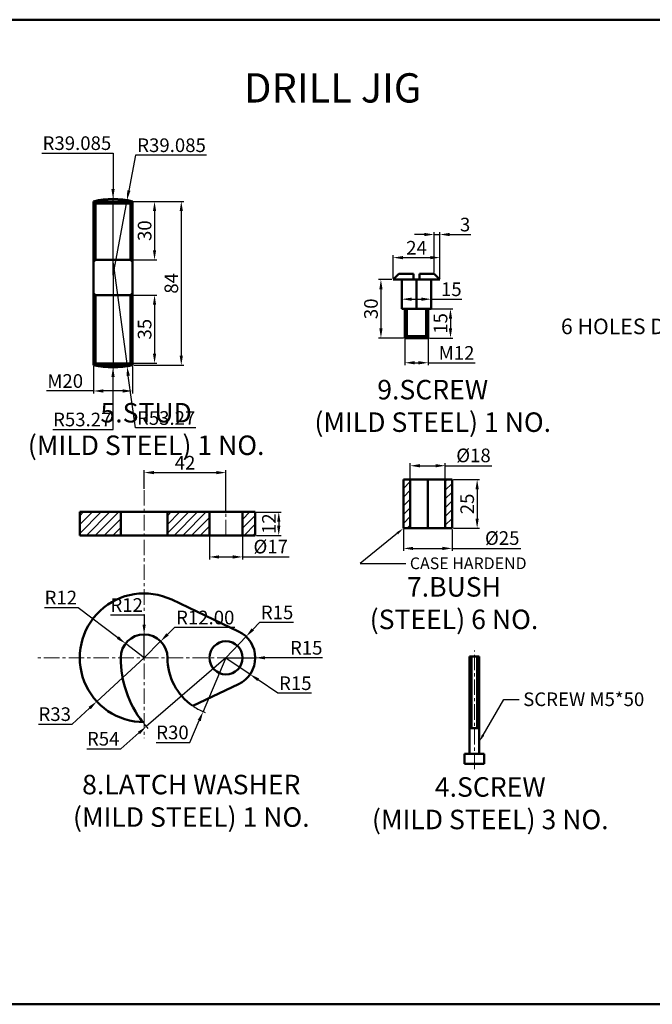
# Model space of a CAD drawing. Units: millimetres. Extents: x 51 to 972, y -225 to 280.
# Tile 2 of 3: x 270 to 594, y -225 to 280. Entities that reach past the tile are written whole.
import ezdxf
from ezdxf import colors
from ezdxf.entities.mleader import LeaderData, LeaderLine
from ezdxf.math import Vec2, Vec3

# ---------------------------------------------------------------- set-up
doc = ezdxf.new("R2010")
doc.units = ezdxf.units.MM
doc.header["$LTSCALE"] = 0.5
doc.linetypes.add('CENTER', pattern=[50.8, 31.75, -6.35, 6.35, -6.35])
for name, color, linetype, lineweight in [('M-CNTR', 1, 'CENTER', 18), ('M-DIMS', 2, 'Continuous', 25), ('M-HATC', 8, 'Continuous', 18), ('M-OUTL', 7, 'Continuous', 50), ('M-TEXT', 7, 'Continuous', 25), ('M-TTLB', 7, 'Continuous', 50)]:
    doc.layers.add(name, color=color, linetype=linetype, lineweight=lineweight)
doc.styles.get("Standard").update_dxf_attribs({"font": 'arial.ttf'})
doc.dimstyles.new('ISO-25', dxfattribs={"dimtxt": 7, "dimasz": 5, "dimexe": 1.25, "dimexo": 0.625, "dimtad": 1, "dimtoh": 1, "dimtxsty": 'Standard', "dimcen": 2.5, "dimadec": 0, "dimazin": 0, "dimtfac": 1, "dimtmove": 0, "dimatfit": 3, "dimfxl": 1, "dimarcsym": 0})

# ---------------------------------------------------------------- blocks, each defined once
blk = doc.blocks.new('*D9')
at = {"layer": 'Defpoints', "color": 0, "ltscale": 0.5, "transparency": 16777216}
for p in [(327.79, 186.58), (327.79, 102.58), (352.8, 102.58)]:
    blk.add_point(p, dxfattribs=at)
at = {"layer": 'M-DIMS', "color": 0, "lineweight": -2, "ltscale": 0.5, "transparency": 16777216}
for p, q in [((328.41, 186.58), (354.05, 186.58)), ((352.8, 181.58), (352.8, 107.58)), ((328.41, 102.58), (354.05, 102.58))]:
    blk.add_line(p, q, dxfattribs=at)
at = {"layer": 'M-DIMS', "color": 0, "ltscale": 0.5, "transparency": 16777216}
for points in [[(351.96, 181.58), (353.63, 181.58), (352.8, 186.58)], [(351.96, 107.58), (353.63, 107.58), (352.8, 102.58)]]:
    blk.add_solid(points, dxfattribs=at)
at = {"layer": 'M-DIMS', "color": 0, "ltscale": 0.5, "transparency": 16777216, "insert": (348.6, 144.58), "char_height": 7, "attachment_point": 5, "rotation": 90}
blk.add_mtext('84', dxfattribs=at)
blk = doc.blocks.new('*D10')
at = {"layer": 'Defpoints', "color": 0, "ltscale": 0.5, "transparency": 16777216}
for p in [(324.33, 138.58), (321.83, 103.58), (339.08, 103.58)]:
    blk.add_point(p, dxfattribs=at)
at = {"layer": 'M-DIMS', "color": 0, "lineweight": -2, "ltscale": 0.5, "transparency": 16777216}
for p, q in [((324.96, 138.58), (340.33, 138.58)), ((339.08, 133.58), (339.08, 108.58)), ((322.46, 103.58), (340.33, 103.58))]:
    blk.add_line(p, q, dxfattribs=at)
at = {"layer": 'M-DIMS', "color": 0, "ltscale": 0.5, "transparency": 16777216}
for points in [[(338.25, 133.58), (339.91, 133.58), (339.08, 138.58)], [(338.25, 108.58), (339.91, 108.58), (339.08, 103.58)]]:
    blk.add_solid(points, dxfattribs=at)
at = {"layer": 'M-DIMS', "color": 0, "ltscale": 0.5, "transparency": 16777216, "insert": (334.88, 121.08), "char_height": 7, "attachment_point": 5, "rotation": 90}
blk.add_mtext('35', dxfattribs=at)
blk = doc.blocks.new('*D11')
at = {"layer": 'Defpoints', "color": 0, "ltscale": 0.5, "transparency": 16777216}
for p in [(317.79, 186.58), (317.79, 156.58), (339.08, 156.58)]:
    blk.add_point(p, dxfattribs=at)
at = {"layer": 'M-DIMS', "color": 0, "lineweight": -2, "ltscale": 0.5, "transparency": 16777216}
for p, q in [((318.41, 186.58), (340.33, 186.58)), ((339.08, 181.58), (339.08, 161.58)), ((318.41, 156.58), (340.33, 156.58))]:
    blk.add_line(p, q, dxfattribs=at)
at = {"layer": 'M-DIMS', "color": 0, "ltscale": 0.5, "transparency": 16777216}
for points in [[(338.25, 181.58), (339.91, 181.58), (339.08, 186.58)], [(338.25, 161.58), (339.91, 161.58), (339.08, 156.58)]]:
    blk.add_solid(points, dxfattribs=at)
at = {"layer": 'M-DIMS', "color": 0, "ltscale": 0.5, "transparency": 16777216, "insert": (334.88, 171.58), "char_height": 7, "attachment_point": 5, "rotation": 90}
blk.add_mtext('30', dxfattribs=at)
blk = doc.blocks.new('*D12')
at = {"layer": 'Defpoints', "color": 0, "ltscale": 0.5, "transparency": 16777216}
for p in [(307.79, 102.58), (327.79, 102.58), (327.79, 89.41)]:
    blk.add_point(p, dxfattribs=at)
at = {"layer": 'M-DIMS', "color": 0, "lineweight": -2, "ltscale": 0.5, "transparency": 16777216}
for p, q in [((307.79, 101.95), (307.79, 88.16)), ((327.79, 101.95), (327.79, 88.16)), ((307.79, 89.41), (283.71, 89.41)), ((322.79, 89.41), (312.79, 89.41))]:
    blk.add_line(p, q, dxfattribs=at)
at = {"layer": 'M-DIMS', "color": 0, "ltscale": 0.5, "transparency": 16777216}
for points in [[(312.79, 90.24), (312.79, 88.57), (307.79, 89.41)], [(322.79, 90.24), (322.79, 88.57), (327.79, 89.41)]]:
    blk.add_solid(points, dxfattribs=at)
at = {"layer": 'M-DIMS', "color": 0, "ltscale": 0.5, "transparency": 16777216, "insert": (293.25, 93.61), "char_height": 7, "attachment_point": 5}
blk.add_mtext('M20', dxfattribs=at)
blk = doc.blocks.new('*D13')
at = {"layer": 'Defpoints', "color": 0, "ltscale": 0.5, "transparency": 16777216}
for p in [(375.73, -47.35), (388.11, -55.82)]:
    blk.add_point(p, dxfattribs=at)
at = {"layer": 'M-DIMS', "color": 0, "lineweight": -2, "ltscale": 0.5, "transparency": 16777216}
for p, q in [((375.73, -47.35), (388.11, -55.82)), ((402.26, -65.5), (392.23, -58.64)), ((419.67, -65.5), (402.26, -65.5))]:
    blk.add_line(p, q, dxfattribs=at)
at = {"layer": 'M-DIMS', "color": 0, "ltscale": 0.5, "transparency": 16777216}
blk.add_solid([(392.71, -57.96), (391.76, -59.33), (388.11, -55.82)], dxfattribs=at)
at = {"layer": 'M-DIMS', "color": 0, "ltscale": 0.5, "transparency": 16777216, "insert": (411.28, -61.3), "char_height": 7, "attachment_point": 5}
blk.add_mtext('R15', dxfattribs=at)
blk = doc.blocks.new('*D14')
at = {"layer": 'Defpoints', "color": 0, "ltscale": 0.5, "transparency": 16777216}
for p in [(324.19, -40.06), (333.73, -47.35)]:
    blk.add_point(p, dxfattribs=at)
at = {"layer": 'M-DIMS', "color": 0, "lineweight": -2, "ltscale": 0.5, "transparency": 16777216}
for p, q in [((282.68, -21.53), (299.96, -21.53)), ((299.96, -21.53), (320.22, -37.03)), ((333.73, -47.35), (324.19, -40.06))]:
    blk.add_line(p, q, dxfattribs=at)
at = {"layer": 'M-DIMS', "color": 0, "ltscale": 0.5, "transparency": 16777216}
blk.add_solid([(320.73, -36.36), (319.72, -37.69), (324.19, -40.06)], dxfattribs=at)
at = {"layer": 'M-DIMS', "color": 0, "ltscale": 0.5, "transparency": 16777216, "insert": (291.01, -17.39), "char_height": 7, "attachment_point": 5}
blk.add_mtext('R12', dxfattribs=at)
blk = doc.blocks.new('*D15')
at = {"layer": 'Defpoints', "color": 0, "ltscale": 0.5, "transparency": 16777216}
for p in [(333.73, -47.35), (309.47, -69.73)]:
    blk.add_point(p, dxfattribs=at)
at = {"layer": 'M-DIMS', "color": 0, "lineweight": -2, "ltscale": 0.5, "transparency": 16777216}
for p, q in [((333.73, -47.35), (309.47, -69.73)), ((296.86, -81.36), (305.8, -73.12)), ((279.51, -81.36), (296.86, -81.36))]:
    blk.add_line(p, q, dxfattribs=at)
at = {"layer": 'M-DIMS', "color": 0, "ltscale": 0.5, "transparency": 16777216}
blk.add_solid([(305.23, -72.51), (306.36, -73.73), (309.47, -69.73)], dxfattribs=at)
at = {"layer": 'M-DIMS', "color": 0, "ltscale": 0.5, "transparency": 16777216, "insert": (287.88, -77.16), "char_height": 7, "attachment_point": 5}
blk.add_mtext('R33', dxfattribs=at)
blk = doc.blocks.new('*D16')
at = {"layer": 'Defpoints', "color": 0, "ltscale": 0.5, "transparency": 16777216}
for p in [(375.73, -47.35), (363.97, -74.95)]:
    blk.add_point(p, dxfattribs=at)
at = {"layer": 'M-DIMS', "color": 0, "lineweight": -2, "ltscale": 0.5, "transparency": 16777216}
for p, q in [((375.73, -47.35), (363.97, -74.95)), ((357.25, -90.73), (362.01, -79.55)), ((339.92, -90.73), (357.25, -90.73))]:
    blk.add_line(p, q, dxfattribs=at)
blk.add_arc((375.73, -47.35), 30, 236.5706, 249.317, dxfattribs=at)
at = {"layer": 'M-DIMS', "color": 0, "ltscale": 0.5, "transparency": 16777216}
blk.add_solid([(361.24, -79.23), (362.78, -79.88), (363.97, -74.95)], dxfattribs=at)
at = {"layer": 'M-DIMS', "color": 0, "ltscale": 0.5, "transparency": 16777216, "insert": (348.27, -86.53), "char_height": 7, "attachment_point": 5}
blk.add_mtext('R30', dxfattribs=at)
blk = doc.blocks.new('*D17')
at = {"layer": 'Defpoints', "color": 0, "ltscale": 0.5, "transparency": 16777216}
for p in [(375.73, -47.35), (334.84, -82.63)]:
    blk.add_point(p, dxfattribs=at)
at = {"layer": 'M-DIMS', "color": 0, "lineweight": -2, "ltscale": 0.5, "transparency": 16777216}
for p, q in [((375.73, -47.35), (334.84, -82.63)), ((321.72, -93.95), (331.06, -85.9)), ((304.4, -93.95), (321.72, -93.95))]:
    blk.add_line(p, q, dxfattribs=at)
blk.add_arc((375.73, -47.35), 54, 218.3216, 222.1171, dxfattribs=at)
at = {"layer": 'M-DIMS', "color": 0, "ltscale": 0.5, "transparency": 16777216}
blk.add_solid([(330.51, -85.27), (331.6, -86.53), (334.84, -82.63)], dxfattribs=at)
at = {"layer": 'M-DIMS', "color": 0, "ltscale": 0.5, "transparency": 16777216, "insert": (312.75, -89.77), "char_height": 7, "attachment_point": 5}
blk.add_mtext('R54', dxfattribs=at)
blk = doc.blocks.new('*D18')
at = {"layer": 'Defpoints', "color": 0, "ltscale": 0.5, "transparency": 16777216}
for p in [(390.73, 27.37), (390.73, 15.37), (402.8, 15.37)]:
    blk.add_point(p, dxfattribs=at)
at = {"layer": 'M-DIMS', "color": 0, "lineweight": -2, "ltscale": 0.5, "transparency": 16777216}
for p, q in [((391.35, 27.37), (404.05, 27.37)), ((402.8, 22.37), (402.8, 20.37)), ((391.35, 15.37), (404.05, 15.37))]:
    blk.add_line(p, q, dxfattribs=at)
at = {"layer": 'M-DIMS', "color": 0, "ltscale": 0.5, "transparency": 16777216}
for points in [[(401.96, 22.37), (403.63, 22.37), (402.8, 27.37)], [(401.96, 20.37), (403.63, 20.37), (402.8, 15.37)]]:
    blk.add_solid(points, dxfattribs=at)
at = {"layer": 'M-DIMS', "color": 0, "ltscale": 0.5, "transparency": 16777216, "insert": (398.66, 21.37), "char_height": 7, "attachment_point": 5, "rotation": 90}
blk.add_mtext('12', dxfattribs=at)
blk = doc.blocks.new('*D19')
at = {"layer": 'Defpoints', "color": 0, "ltscale": 0.5, "transparency": 16777216}
for p in [(367.23, 15.37), (384.23, 15.37), (384.23, 4.33)]:
    blk.add_point(p, dxfattribs=at)
at = {"layer": 'M-DIMS', "color": 0, "lineweight": -2, "ltscale": 0.5, "transparency": 16777216}
for p, q in [((367.23, 14.75), (367.23, 3.08)), ((384.23, 14.75), (384.23, 3.08)), ((372.23, 4.33), (379.23, 4.33)), ((384.23, 4.33), (408.12, 4.33))]:
    blk.add_line(p, q, dxfattribs=at)
at = {"layer": 'M-DIMS', "color": 0, "ltscale": 0.5, "transparency": 16777216}
for points in [[(372.23, 5.17), (372.23, 3.5), (367.23, 4.33)], [(379.23, 5.17), (379.23, 3.5), (384.23, 4.33)]]:
    blk.add_solid(points, dxfattribs=at)
at = {"layer": 'M-DIMS', "color": 0, "ltscale": 0.5, "transparency": 16777216, "insert": (398.67, 8.73), "char_height": 7, "attachment_point": 5}
blk.add_mtext('%%C17', dxfattribs=at)
blk = doc.blocks.new('*D28')
at = {"layer": 'Defpoints', "color": 0, "ltscale": 0.5, "transparency": 16777216}
for p in [(485.47, 157.77), (461.47, 146.53), (485.47, 146.53)]:
    blk.add_point(p, dxfattribs=at)
at = {"layer": 'M-DIMS', "color": 0, "lineweight": -2, "ltscale": 0.5, "transparency": 16777216}
for p, q in [((461.47, 147.15), (461.47, 159.02)), ((466.47, 157.77), (480.47, 157.77)), ((485.47, 147.15), (485.47, 159.02))]:
    blk.add_line(p, q, dxfattribs=at)
at = {"layer": 'M-DIMS', "color": 0, "ltscale": 0.5, "transparency": 16777216}
for points in [[(466.47, 158.6), (466.47, 156.94), (461.47, 157.77)], [(480.47, 158.6), (480.47, 156.94), (485.47, 157.77)]]:
    blk.add_solid(points, dxfattribs=at)
at = {"layer": 'M-DIMS', "color": 0, "ltscale": 0.5, "transparency": 16777216, "insert": (473.47, 161.91), "char_height": 7, "attachment_point": 5}
blk.add_mtext('24', dxfattribs=at)
blk = doc.blocks.new('*D29')
at = {"layer": 'Defpoints', "color": 0, "ltscale": 0.5, "transparency": 16777216}
for p in [(461.47, 146.53), (455.21, 116.53), (467.47, 116.53)]:
    blk.add_point(p, dxfattribs=at)
at = {"layer": 'M-DIMS', "color": 0, "lineweight": -2, "ltscale": 0.5, "transparency": 16777216}
for p, q in [((460.84, 146.53), (453.96, 146.53)), ((455.21, 141.53), (455.21, 121.53)), ((466.84, 116.53), (453.96, 116.53))]:
    blk.add_line(p, q, dxfattribs=at)
at = {"layer": 'M-DIMS', "color": 0, "ltscale": 0.5, "transparency": 16777216}
for points in [[(454.38, 141.53), (456.05, 141.53), (455.21, 146.53)], [(454.38, 121.53), (456.05, 121.53), (455.21, 116.53)]]:
    blk.add_solid(points, dxfattribs=at)
at = {"layer": 'M-DIMS', "color": 0, "ltscale": 0.5, "transparency": 16777216, "insert": (451.01, 131.53), "char_height": 7, "attachment_point": 5, "rotation": 90}
blk.add_mtext('30', dxfattribs=at)
blk = doc.blocks.new('*D30')
at = {"layer": 'Defpoints', "color": 0, "ltscale": 0.5, "transparency": 16777216}
for p in [(465.97, 146.53), (480.97, 146.53), (480.97, 136.45)]:
    blk.add_point(p, dxfattribs=at)
at = {"layer": 'M-DIMS', "color": 0, "lineweight": -2, "ltscale": 0.5, "transparency": 16777216}
for p, q in [((465.97, 145.9), (465.97, 135.2)), ((480.97, 145.9), (480.97, 135.2)), ((470.97, 136.45), (475.97, 136.45)), ((480.97, 136.45), (496.64, 136.45))]:
    blk.add_line(p, q, dxfattribs=at)
at = {"layer": 'M-DIMS', "color": 0, "ltscale": 0.5, "transparency": 16777216}
for points in [[(470.97, 137.28), (470.97, 135.62), (465.97, 136.45)], [(475.97, 137.28), (475.97, 135.62), (480.97, 136.45)]]:
    blk.add_solid(points, dxfattribs=at)
at = {"layer": 'M-DIMS', "color": 0, "ltscale": 0.5, "transparency": 16777216, "insert": (491.3, 140.65), "char_height": 7, "attachment_point": 5}
blk.add_mtext('15', dxfattribs=at)
blk = doc.blocks.new('*D31')
at = {"layer": 'Defpoints', "color": 0, "ltscale": 0.5, "transparency": 16777216}
for p in [(485.47, 169.6), (482.47, 149.53), (485.47, 146.53)]:
    blk.add_point(p, dxfattribs=at)
at = {"layer": 'M-DIMS', "color": 0, "lineweight": -2, "ltscale": 0.5, "transparency": 16777216}
for p, q in [((477.47, 169.6), (472.47, 169.6)), ((482.47, 150.15), (482.47, 170.85)), ((482.47, 169.6), (485.47, 169.6)), ((485.47, 147.15), (485.47, 170.85)), ((490.47, 169.6), (501.3, 169.6))]:
    blk.add_line(p, q, dxfattribs=at)
at = {"layer": 'M-DIMS', "color": 0, "ltscale": 0.5, "transparency": 16777216}
for points in [[(477.47, 170.43), (477.47, 168.76), (482.47, 169.6)], [(490.47, 170.43), (490.47, 168.76), (485.47, 169.6)]]:
    blk.add_solid(points, dxfattribs=at)
at = {"layer": 'M-DIMS', "color": 0, "ltscale": 0.5, "transparency": 16777216, "insert": (498.39, 173.8), "char_height": 7, "attachment_point": 5}
blk.add_mtext('3', dxfattribs=at)
blk = doc.blocks.new('*D32')
at = {"layer": 'Defpoints', "color": 0, "ltscale": 0.5, "transparency": 16777216}
for p in [(467.47, 117.53), (479.47, 117.53), (479.47, 103.87)]:
    blk.add_point(p, dxfattribs=at)
at = {"layer": 'M-DIMS', "color": 0, "lineweight": -2, "ltscale": 0.5, "transparency": 16777216}
for p, q in [((467.47, 116.9), (467.47, 102.62)), ((479.47, 116.9), (479.47, 102.62)), ((472.47, 103.87), (474.47, 103.87)), ((479.47, 103.87), (503.5, 103.87))]:
    blk.add_line(p, q, dxfattribs=at)
at = {"layer": 'M-DIMS', "color": 0, "ltscale": 0.5, "transparency": 16777216}
for points in [[(472.47, 104.7), (472.47, 103.03), (467.47, 103.87)], [(474.47, 104.7), (474.47, 103.03), (479.47, 103.87)]]:
    blk.add_solid(points, dxfattribs=at)
at = {"layer": 'M-DIMS', "color": 0, "ltscale": 0.5, "transparency": 16777216, "insert": (493.99, 108.01), "char_height": 7, "attachment_point": 5}
blk.add_mtext('M12', dxfattribs=at)
blk = doc.blocks.new('*D33')
at = {"layer": 'Defpoints', "color": 0, "ltscale": 0.5, "transparency": 16777216}
for p in [(479.47, 131.53), (479.47, 116.53), (490.89, 116.53)]:
    blk.add_point(p, dxfattribs=at)
at = {"layer": 'M-DIMS', "color": 0, "lineweight": -2, "ltscale": 0.5, "transparency": 16777216}
for p, q in [((480.09, 131.53), (492.14, 131.53)), ((490.89, 126.53), (490.89, 121.53)), ((480.09, 116.53), (492.14, 116.53))]:
    blk.add_line(p, q, dxfattribs=at)
at = {"layer": 'M-DIMS', "color": 0, "ltscale": 0.5, "transparency": 16777216}
for points in [[(490.05, 126.53), (491.72, 126.53), (490.89, 131.53)], [(490.05, 121.53), (491.72, 121.53), (490.89, 116.53)]]:
    blk.add_solid(points, dxfattribs=at)
at = {"layer": 'M-DIMS', "color": 0, "ltscale": 0.5, "transparency": 16777216, "insert": (486.69, 124.03), "char_height": 7, "attachment_point": 5, "rotation": 90}
blk.add_mtext('15', dxfattribs=at)
blk = doc.blocks.new('*D34')
at = {"layer": 'Defpoints', "color": 0, "ltscale": 0.5, "transparency": 16777216}
for p in [(491.74, 44.01), (491.74, 19.01), (504.56, 19.01)]:
    blk.add_point(p, dxfattribs=at)
at = {"layer": 'M-DIMS', "color": 0, "lineweight": -2, "ltscale": 0.5, "transparency": 16777216}
for p, q in [((492.37, 44.01), (505.81, 44.01)), ((504.56, 39.01), (504.56, 24.01)), ((492.37, 19.01), (505.81, 19.01))]:
    blk.add_line(p, q, dxfattribs=at)
at = {"layer": 'M-DIMS', "color": 0, "ltscale": 0.5, "transparency": 16777216}
for points in [[(503.72, 39.01), (505.39, 39.01), (504.56, 44.01)], [(503.72, 24.01), (505.39, 24.01), (504.56, 19.01)]]:
    blk.add_solid(points, dxfattribs=at)
at = {"layer": 'M-DIMS', "color": 0, "ltscale": 0.5, "transparency": 16777216, "insert": (500.36, 31.51), "char_height": 7, "attachment_point": 5, "rotation": 90}
blk.add_mtext('25', dxfattribs=at)
blk = doc.blocks.new('*D35')
at = {"layer": 'Defpoints', "color": 0, "ltscale": 0.5, "transparency": 16777216}
for p in [(488.24, 51.09), (470.24, 44.01), (488.24, 44.01)]:
    blk.add_point(p, dxfattribs=at)
at = {"layer": 'M-DIMS', "color": 0, "lineweight": -2, "ltscale": 0.5, "transparency": 16777216}
for p, q in [((470.24, 44.63), (470.24, 52.34)), ((475.24, 51.09), (483.24, 51.09)), ((488.24, 44.63), (488.24, 52.34)), ((488.24, 51.09), (512.15, 51.09))]:
    blk.add_line(p, q, dxfattribs=at)
at = {"layer": 'M-DIMS', "color": 0, "ltscale": 0.5, "transparency": 16777216}
for points in [[(475.24, 51.92), (475.24, 50.25), (470.24, 51.09)], [(483.24, 51.92), (483.24, 50.25), (488.24, 51.09)]]:
    blk.add_solid(points, dxfattribs=at)
at = {"layer": 'M-DIMS', "color": 0, "ltscale": 0.5, "transparency": 16777216, "insert": (502.69, 55.48), "char_height": 7, "attachment_point": 5}
blk.add_mtext('%%C18', dxfattribs=at)
blk = doc.blocks.new('*D36')
at = {"layer": 'Defpoints', "color": 0, "ltscale": 0.5, "transparency": 16777216}
for p in [(466.74, 19.01), (491.74, 19.01), (491.74, 8.7)]:
    blk.add_point(p, dxfattribs=at)
at = {"layer": 'M-DIMS', "color": 0, "lineweight": -2, "ltscale": 0.5, "transparency": 16777216}
for p, q in [((466.74, 18.38), (466.74, 7.45)), ((491.74, 18.38), (491.74, 7.45)), ((471.74, 8.7), (486.74, 8.7)), ((491.74, 8.7), (526.9, 8.7))]:
    blk.add_line(p, q, dxfattribs=at)
at = {"layer": 'M-DIMS', "color": 0, "ltscale": 0.5, "transparency": 16777216}
for points in [[(471.74, 9.54), (471.74, 7.87), (466.74, 8.7)], [(486.74, 9.54), (486.74, 7.87), (491.74, 8.7)]]:
    blk.add_solid(points, dxfattribs=at)
at = {"layer": 'M-DIMS', "color": 0, "ltscale": 0.5, "transparency": 16777216, "insert": (517.43, 13.1), "char_height": 7, "attachment_point": 5}
blk.add_mtext('%%C25', dxfattribs=at)
blk = doc.blocks.new('*D46')
at = {"layer": 'Defpoints', "color": 0, "ltscale": 0.5, "transparency": 16777216}
for p in [(375.73, 47.57), (333.73, 38.57), (375.73, 27.37)]:
    blk.add_point(p, dxfattribs=at)
at = {"layer": 'M-DIMS', "color": 0, "lineweight": -2, "ltscale": 0.5, "transparency": 16777216}
for p, q in [((333.73, 39.2), (333.73, 48.82)), ((338.73, 47.57), (370.73, 47.57)), ((375.73, 28), (375.73, 48.82))]:
    blk.add_line(p, q, dxfattribs=at)
at = {"layer": 'M-DIMS', "color": 0, "ltscale": 0.5, "transparency": 16777216}
for points in [[(338.73, 48.41), (338.73, 46.74), (333.73, 47.57)], [(370.73, 48.41), (370.73, 46.74), (375.73, 47.57)]]:
    blk.add_solid(points, dxfattribs=at)
at = {"layer": 'M-DIMS', "color": 0, "ltscale": 0.5, "transparency": 16777216, "insert": (354.73, 51.71), "char_height": 7, "attachment_point": 5}
blk.add_mtext('42', dxfattribs=at)
blk = doc.blocks.new('*D48')
at = {"layer": 'Defpoints', "color": 0, "ltscale": 0.5, "transparency": 16777216}
for p in [(333.73, -35.35), (333.73, -47.35)]:
    blk.add_point(p, dxfattribs=at)
at = {"layer": 'M-DIMS', "color": 0, "lineweight": -2, "ltscale": 0.5, "transparency": 16777216}
for p, q in [((316.45, -25.35), (333.73, -25.35)), ((333.73, -25.35), (333.73, -30.35)), ((333.73, -47.35), (333.73, -35.35))]:
    blk.add_line(p, q, dxfattribs=at)
at = {"layer": 'M-DIMS', "color": 0, "ltscale": 0.5, "transparency": 16777216}
blk.add_solid([(334.56, -30.35), (332.89, -30.35), (333.73, -35.35)], dxfattribs=at)
at = {"layer": 'M-DIMS', "color": 0, "ltscale": 0.5, "transparency": 16777216, "insert": (324.77, -21.21), "char_height": 7, "attachment_point": 5}
blk.add_mtext('R12', dxfattribs=at)
blk = doc.blocks.new('*D49')
at = {"layer": 'Defpoints', "color": 0, "ltscale": 0.5, "transparency": 16777216}
for p in [(375.73, -47.35), (390.73, -47.35)]:
    blk.add_point(p, dxfattribs=at)
at = {"layer": 'M-DIMS', "color": 0, "lineweight": -2, "ltscale": 0.5, "transparency": 16777216}
for p, q in [((375.73, -47.35), (390.73, -47.35)), ((407.87, -47.35), (395.73, -47.35)), ((425.28, -47.35), (407.87, -47.35))]:
    blk.add_line(p, q, dxfattribs=at)
at = {"layer": 'M-DIMS', "color": 0, "ltscale": 0.5, "transparency": 16777216}
blk.add_solid([(395.73, -46.52), (395.73, -48.19), (390.73, -47.35)], dxfattribs=at)
at = {"layer": 'M-DIMS', "color": 0, "ltscale": 0.5, "transparency": 16777216, "insert": (416.89, -43.15), "char_height": 7, "attachment_point": 5}
blk.add_mtext('R15', dxfattribs=at)
blk = doc.blocks.new('*D50')
at = {"layer": 'Defpoints', "color": 0, "ltscale": 0.5, "transparency": 16777216}
for p in [(317.79, 154.9), (317.79, 101.63)]:
    blk.add_point(p, dxfattribs=at)
at = {"layer": 'M-DIMS', "color": 0, "lineweight": -2, "ltscale": 0.5, "transparency": 16777216}
for p, q in [((317.79, 154.9), (317.79, 101.63)), ((317.79, 69.67), (317.79, 96.63)), ((286.84, 69.67), (317.79, 69.67))]:
    blk.add_line(p, q, dxfattribs=at)
at = {"layer": 'M-DIMS', "color": 0, "ltscale": 0.5, "transparency": 16777216}
blk.add_solid([(316.96, 96.63), (318.62, 96.63), (317.79, 101.63)], dxfattribs=at)
at = {"layer": 'M-DIMS', "color": 0, "ltscale": 0.5, "transparency": 16777216, "insert": (302, 73.87), "char_height": 7, "attachment_point": 5}
blk.add_mtext('R53.27', dxfattribs=at)
blk = doc.blocks.new('*D51')
at = {"layer": 'Defpoints', "color": 0, "ltscale": 0.5, "transparency": 16777216}
for p in [(317.79, 187.88), (317.79, 148.79)]:
    blk.add_point(p, dxfattribs=at)
at = {"layer": 'M-DIMS', "color": 0, "lineweight": -2, "ltscale": 0.5, "transparency": 16777216}
for p, q in [((281.35, 211.33), (317.79, 211.33)), ((317.79, 211.33), (317.79, 192.88)), ((317.79, 148.79), (317.79, 187.88))]:
    blk.add_line(p, q, dxfattribs=at)
at = {"layer": 'M-DIMS', "color": 0, "ltscale": 0.5, "transparency": 16777216}
blk.add_solid([(318.62, 192.88), (316.96, 192.88), (317.79, 187.88)], dxfattribs=at)
at = {"layer": 'M-DIMS', "color": 0, "ltscale": 0.5, "transparency": 16777216, "insert": (299.26, 215.53), "char_height": 7, "attachment_point": 5}
blk.add_mtext('R39.085', dxfattribs=at)
blk = doc.blocks.new('*D58')
at = {"layer": 'Defpoints', "color": 0, "ltscale": 0.5, "transparency": 16777216}
for p in [(386.04, -36.46), (375.73, -47.35)]:
    blk.add_point(p, dxfattribs=at)
at = {"layer": 'M-DIMS', "color": 0, "lineweight": -2, "ltscale": 0.5, "transparency": 16777216}
for p, q in [((392.91, -29.2), (389.48, -32.83)), ((410.32, -29.2), (392.91, -29.2)), ((375.73, -47.35), (386.04, -36.46))]:
    blk.add_line(p, q, dxfattribs=at)
at = {"layer": 'M-DIMS', "color": 0, "ltscale": 0.5, "transparency": 16777216}
blk.add_solid([(388.87, -32.26), (390.08, -33.4), (386.04, -36.46)], dxfattribs=at)
at = {"layer": 'M-DIMS', "color": 0, "ltscale": 0.5, "transparency": 16777216, "insert": (401.93, -25), "char_height": 7, "attachment_point": 5}
blk.add_mtext('R15', dxfattribs=at)
blk = doc.blocks.new('*D61')
at = {"layer": 'Defpoints', "color": 0, "ltscale": 0.5, "transparency": 16777216}
for p in [(342.22, -38.88), (333.73, -47.35)]:
    blk.add_point(p, dxfattribs=at)
at = {"layer": 'M-DIMS', "color": 0, "lineweight": -2, "ltscale": 0.5, "transparency": 16777216}
for p, q in [((349.3, -31.82), (345.76, -35.35)), ((380.22, -31.82), (349.3, -31.82)), ((333.73, -47.35), (342.22, -38.88))]:
    blk.add_line(p, q, dxfattribs=at)
at = {"layer": 'M-DIMS', "color": 0, "ltscale": 0.5, "transparency": 16777216}
blk.add_solid([(345.17, -34.76), (346.35, -35.94), (342.22, -38.88)], dxfattribs=at)
at = {"layer": 'M-DIMS', "color": 0, "ltscale": 0.5, "transparency": 16777216, "insert": (365.08, -27.62), "char_height": 7, "attachment_point": 5}
blk.add_mtext('R12.00', dxfattribs=at)
blk = doc.blocks.new('*D62')
at = {"layer": 'Defpoints', "color": 0, "ltscale": 0.5, "transparency": 16777216}
for p in [(324.97, 187.21), (317.79, 148.79)]:
    blk.add_point(p, dxfattribs=at)
at = {"layer": 'M-DIMS', "color": 0, "lineweight": -2, "ltscale": 0.5, "transparency": 16777216}
for p, q in [((329.27, 210.27), (325.88, 192.13)), ((365.71, 210.27), (329.27, 210.27)), ((317.79, 148.79), (324.97, 187.21))]:
    blk.add_line(p, q, dxfattribs=at)
at = {"layer": 'M-DIMS', "color": 0, "ltscale": 0.5, "transparency": 16777216}
blk.add_solid([(325.06, 192.28), (326.7, 191.98), (324.97, 187.21)], dxfattribs=at)
at = {"layer": 'M-DIMS', "color": 0, "ltscale": 0.5, "transparency": 16777216, "insert": (347.8, 214.47), "char_height": 7, "attachment_point": 5}
blk.add_mtext('R39.085', dxfattribs=at)
blk = doc.blocks.new('*D63')
at = {"layer": 'Defpoints', "color": 0, "ltscale": 0.5, "transparency": 16777216}
for p in [(317.79, 154.9), (324.96, 102.11)]:
    blk.add_point(p, dxfattribs=at)
at = {"layer": 'M-DIMS', "color": 0, "lineweight": -2, "ltscale": 0.5, "transparency": 16777216}
for p, q in [((317.79, 154.9), (324.96, 102.11)), ((329.26, 70.44), (325.63, 97.16)), ((360.2, 70.44), (329.26, 70.44))]:
    blk.add_line(p, q, dxfattribs=at)
at = {"layer": 'M-DIMS', "color": 0, "ltscale": 0.5, "transparency": 16777216}
blk.add_solid([(326.46, 97.27), (324.8, 97.05), (324.96, 102.11)], dxfattribs=at)
at = {"layer": 'M-DIMS', "color": 0, "ltscale": 0.5, "transparency": 16777216, "insert": (345.04, 74.65), "char_height": 7, "attachment_point": 5}
blk.add_mtext('R53.27', dxfattribs=at)

msp = doc.modelspace()

# ---------------------------------------------------------------- hatches: boundary and pattern name
at = {"layer": 'M-HATC', "ltscale": 0.5}
h = msp.add_hatch(dxfattribs=at)
h.set_pattern_fill('ANSI31', color=256)
h.set_pattern_definition([(45, (0, 26.255), (-2.245064, 2.245064), [])])
h.paths.add_polyline_path([(470.2408, 44.0072), (466.7408, 44.0072), (466.7408, 19.0072), (470.2408, 19.0072)])
h.paths.add_polyline_path([(491.7408, 44.0072), (488.2408, 44.0072), (488.2408, 19.0072), (491.7408, 19.0072)])
h = msp.add_hatch(dxfattribs=at)
h.set_pattern_fill('ANSI31', color=256)
h.set_pattern_definition([(45, (-188.987, -356.5694), (-2.245064, 2.245064), [])])
h.paths.add_polyline_path([(300.7264, 27.375), (300.7264, 15.375), (321.7264, 15.375), (321.7264, 27.375)])
h.paths.add_polyline_path([(367.2264, 15.375), (367.2264, 27.375), (345.7264, 27.375), (345.7264, 15.375)])
h.paths.add_polyline_path([(384.2264, 15.375), (390.7264, 15.375), (390.7264, 27.375), (384.2264, 27.375)])

# ---------------------------------------------------------------- linework, layer by layer
at = {"layer": 'M-CNTR'}
msp.add_line((317.7891, 191.1627), (317.7891, 98.9413), dxfattribs=at)
at = {"layer": 'M-CNTR', "ltscale": 0.5}
for p, q in [((333.7264, 38.5724), (333.7264, -88.5788)), ((375.7264, 15.375), (375.7264, 27.375)), ((503.1325, -104.529), (503.1325, -43.6952)), ((417.2939, -47.3528), (278.7392, -47.3528))]:
    msp.add_line(p, q, dxfattribs=at)
at = {"layer": 'M-OUTL'}
for p, q in [((307.7891, 186.5769), (327.7891, 186.5769)), ((307.7891, 155.5769), (307.7891, 186.5769)), ((307.7891, 185.5769), (327.7891, 185.5769)), ((308.7891, 156.5769), (308.7891, 186.5769)), ((326.7891, 186.5769), (326.7891, 156.5769)), ((327.7891, 186.5769), (327.7891, 155.5769)), ((307.7891, 155.5769), (308.7891, 156.5769)), ((308.7891, 156.5769), (326.7891, 156.5769)), ((327.7891, 155.5769), (326.7891, 156.5769)), ((307.7891, 139.5769), (307.7891, 155.5769)), ((327.7891, 155.5769), (327.7891, 139.5769)), ((307.7891, 139.5769), (308.7891, 138.5769)), ((307.7891, 139.5769), (307.7891, 102.5769)), ((326.7891, 138.5769), (308.7891, 138.5769)), ((308.7891, 102.5769), (308.7891, 138.5769)), ((327.7891, 139.5769), (326.7891, 138.5769)), ((326.7891, 138.5769), (326.7891, 102.5769)), ((327.7891, 139.5769), (327.7891, 102.5769)), ((327.7891, 103.5769), (307.7891, 103.5769)), ((327.7891, 102.5769), (307.7891, 102.5769))]:
    msp.add_line(p, q, dxfattribs=at)
at = {"layer": 'M-OUTL', "ltscale": 0.5}
for p, q in [((461.4694, 146.5274), (464.4694, 149.5274)), ((485.4694, 146.5274), (461.4694, 146.5274)), ((461.4694, 146.5274), (461.4694, 146.5274)), ((464.4694, 149.5274), (471.9694, 149.5274)), ((465.9694, 146.5274), (465.9694, 131.5274)), ((471.9694, 146.5274), (471.9694, 149.5274)), ((473.4694, 146.5274), (473.4694, 131.5274)), ((474.9694, 146.5274), (474.9694, 149.5274)), ((474.9694, 149.5274), (482.4694, 149.5274)), ((480.9694, 146.5274), (480.9694, 131.5274)), ((485.4694, 146.5274), (482.4694, 149.5274)), ((485.4694, 146.5274), (485.4694, 146.5274)), ((480.9694, 131.5274), (465.9694, 131.5274)), ((467.4694, 116.5274), (467.4694, 131.5274)), ((468.4694, 116.5274), (468.4694, 131.5274)), ((478.4694, 116.5274), (478.4694, 131.5274)), ((479.4694, 116.5274), (479.4694, 131.5274)), ((467.4694, 117.5274), (479.4694, 117.5274)), ((467.4694, 116.5274), (479.4694, 116.5274)), ((466.7408, 44.0072), (491.7408, 44.0072)), ((466.7408, 19.0072), (466.7408, 44.0072)), ((470.2408, 44.0072), (470.2408, 19.0072)), ((479.2408, 44.0072), (479.2408, 19.0072)), ((488.2408, 44.0072), (488.2408, 19.0072)), ((491.7408, 44.0072), (491.7408, 19.0072)), ((390.7264, 27.375), (300.7264, 27.375)), ((300.7264, 27.375), (300.7264, 15.375)), ((321.7264, 15.375), (321.7264, 27.375)), ((345.7264, 15.375), (345.7264, 27.375)), ((367.2264, 15.375), (367.2264, 27.375)), ((384.2264, 15.375), (384.2264, 27.375)), ((390.7264, 15.375), (390.7264, 27.375)), ((300.7264, 15.375), (390.7264, 15.375)), ((491.7408, 19.0072), (466.7408, 19.0072)), ((347.8693, -17.537), (382.155, -33.8002)), ((500.6325, -46.6422), (500.6325, -96.6422)), ((505.6325, -46.6422), (500.6325, -46.6422)), ((501.6325, -46.6422), (501.6325, -83.4304)), ((504.6325, -83.4304), (504.6325, -46.6422)), ((505.6325, -96.6422), (505.6325, -46.6422)), ((358.6812, -72.04), (382.155, -60.9054)), ((500.6325, -83.4304), (505.6325, -83.4304)), ((498.1325, -101.6422), (498.1325, -96.6422)), ((498.1325, -96.6422), (500.6325, -96.6422)), ((500.6325, -96.6422), (505.6325, -96.6422)), ((505.6325, -96.6422), (508.1325, -96.6422)), ((508.1325, -96.6422), (508.1325, -101.6422)), ((508.1325, -101.6422), (498.1325, -101.6422))]:
    msp.add_line(p, q, dxfattribs=at)
msp.add_circle((375.7264, -47.3528), 8.5, dxfattribs=at)
at = {"layer": 'M-OUTL'}
for centre, radius, start, end in [((317.7891, 148.7928), 39.085, 75.175893, 104.824107), ((317.7891, 154.898), 53.2681, 259.179682, 280.820318)]:
    msp.add_arc(centre, radius, start, end, dxfattribs=at)
at = {"layer": 'M-OUTL', "ltscale": 0.5}
for centre, radius, start, end in [((333.7264, -47.3528), 33, 64.623066, 270), ((375.7264, -47.3528), 15, 295.376934, 64.623066), ((333.7264, -47.3528), 12, 0, 180), ((375.7264, -47.3528), 54, 180, 217.658462), ((375.7264, -47.3528), 30, 180, 235.376934)]:
    msp.add_arc(centre, radius, start, end, dxfattribs=at)
at = {"layer": 'M-TTLB', "ltscale": 0.5}
msp.add_lwpolyline([(50.8898, 279.7282), (925.0778, 279.7282), (925.0778, -224.9845), (50.8898, -224.9845)], close=True, dxfattribs=at)

# ---------------------------------------------------------------- texts
at = {"layer": 'M-TEXT', "ltscale": 0.5, "insert": (385.0019, 252.2685), "char_height": 15, "attachment_point": 1}
msp.add_mtext_dynamic_manual_height_columns('DRILL JIG', width=236.31945, gutter_width=12.5, heights=[0], dxfattribs=at)
at = {"layer": 'M-TEXT', "char_height": 10, "attachment_point": 1}
for s, insert in [('\\pxqc;9.SCREW \\P(MILD STEEL) 1 NO. ', (386.0603, 95.0887)), ('\\pxqc;5.STUD \\P(MILD STEEL) 1 NO. ', (239.0678, 83.2518)), ('\\pxqc;7.BUSH \\P(STEEL) 6 NO. ', (396.9728, -5.9937)), ('\\pxqc;8.LATCH WASHER \\P(MILD STEEL) 1 NO. ', (262.2202, -107.3381)), ('\\pxqc;4.SCREW \\P(MILD STEEL) 3 NO. ', (415.5824, -108.579))]:
    msp.add_mtext_dynamic_manual_height_columns(s, width=191.418549, gutter_width=12.5, heights=[0], dxfattribs=dict(at, insert=insert))

# ---------------------------------------------------------------- dimensions: what is measured, and where the dimension line sits
at = {"layer": 'M-DIMS', "ltscale": 0.5}
for center, mpoint, override, picture, middle in [((317.7891, 148.7928), (317.789, 187.8778), {"dimdec": 3, "dimlfac": 1, "dimrnd": 0, "dimzin": 0, "dimdsep": 46, "dimlunit": 2}, '*D51', (299.2581, 211.3288)), ((317.7891, 148.7928), (324.9652, 187.2134), {"dimdec": 3, "dimlfac": 1, "dimrnd": 0, "dimzin": 0, "dimdsep": 46, "dimlunit": 2}, '*D62', (347.8017, 210.2658)), ((317.7891, 154.898), (317.789, 101.6299), {"dimdec": 2, "dimlfac": 1, "dimrnd": 0, "dimzin": 0, "dimdsep": 46, "dimlunit": 2}, '*D50', (302.0036, 69.669)), ((317.7891, 154.898), (324.9573, 102.1144), {"dimdec": 2, "dimlfac": 1, "dimrnd": 0, "dimzin": 0, "dimdsep": 46, "dimlunit": 2}, '*D63', (345.0435, 70.4442)), ((333.7264, -47.3528), (324.1943, -40.0632), {"dimclrd": 0, "dimclre": 0, "dimclrt": 0}, '*D14', (291.0064, -21.5294)), ((375.7264, -47.3528), (334.843, -82.631), {"dimclrd": 0, "dimclre": 0, "dimclrt": 0}, '*D17', (312.7479, -93.9533))]:
    dim = msp.add_radius_dim(center=center, mpoint=mpoint, dimstyle='ISO-25', override=override, dxfattribs=at)
    dim.commit()
    dim.dimension.update_dxf_attribs({"geometry": picture, "text_midpoint": middle, "dimtype": 164})
for base, p1, p2, picture, middle in [((339.0815, 156.5769), (317.7891, 186.5769), (317.7891, 156.5769), '*D11', (334.8801, 171.5769)), ((352.7971, 102.5769), (327.7891, 186.5769), (327.7891, 102.5769), '*D9', (348.5981, 144.5769)), ((455.213, 116.5274), (461.4694, 146.5274), (467.4694, 116.5274), '*D29', (451.0116, 131.5274)), ((339.0815, 103.5769), (324.3333, 138.5769), (321.8336, 103.5769), '*D10', (334.8801, 121.0769)), ((490.8862, 116.5274), (479.4694, 131.5274), (479.4694, 116.5274), '*D33', (486.6872, 124.0274)), ((504.5554, 19.0072), (491.7408, 44.0072), (491.7408, 19.0072), '*D34', (500.3564, 31.5072)), ((402.7953, 15.375), (390.7264, 27.375), (390.7264, 15.375), '*D18', (398.656, 21.375))]:
    dim = msp.add_linear_dim(base=base, p1=p1, p2=p2, angle=90, dimstyle='ISO-25', override={"dimclrd": 0, "dimclre": 0, "dimclrt": 0}, dxfattribs=at)
    dim.commit()
    dim.dimension.update_dxf_attribs({"geometry": picture, "text_midpoint": middle})
for base, p1, p2, override, picture, middle in [((485.4694, 169.5951), (482.4694, 149.5274), (485.4694, 146.5274), {"dimclrd": 0, "dimclre": 0, "dimclrt": 0}, '*D31', (498.3863, 173.7965)), ((485.4694, 157.7701), (461.4694, 146.5274), (485.4694, 146.5274), {"dimclrd": 0, "dimclre": 0, "dimclrt": 0}, '*D28', (473.4694, 161.9094)), ((375.7264, 47.5724), (333.7264, 38.5724), (375.7264, 27.375), {"dimdec": 0, "dimlfac": 1, "dimrnd": 0, "dimzin": 0, "dimdsep": 46, "dimlunit": 2}, '*D46', (354.7264, 51.7118))]:
    dim = msp.add_linear_dim(base=base, p1=p1, p2=p2, dimstyle='ISO-25', override=override, dxfattribs=at)
    dim.commit()
    dim.dimension.update_dxf_attribs({"geometry": picture, "text_midpoint": middle})
dim = msp.add_linear_dim(base=(480.9694, 136.451), p1=(465.9694, 146.5274), p2=(480.9694, 146.5274), dimstyle='ISO-25', override={"dimclrd": 0, "dimclre": 0, "dimclrt": 0}, dxfattribs=at)
dim.commit()
dim.dimension.update_dxf_attribs({"geometry": '*D30', "text_midpoint": (491.3048, 136.451), "dimtype": 160})
for base, p1, p2, text, picture, middle in [((479.4694, 103.8678), (467.4694, 117.5274), (479.4694, 117.5274), 'M<>', '*D32', (493.9852, 103.8678)), ((327.7891, 89.4077), (307.7891, 102.5769), (327.7891, 102.5769), 'M<>', '*D12', (293.2494, 89.4077)), ((491.7408, 8.7039), (466.7408, 19.0072), (491.7408, 19.0072), '%%C<>', '*D36', (517.4308, 8.7039))]:
    dim = msp.add_linear_dim(base=base, p1=p1, p2=p2, text=text, dimstyle='ISO-25', override={"dimclrd": 0, "dimclre": 0, "dimclrt": 0}, dxfattribs=at)
    dim.commit()
    dim.dimension.update_dxf_attribs({"geometry": picture, "text_midpoint": middle, "dimtype": 160})
for base, p1, p2, picture, middle in [((488.2408, 51.0881), (470.2408, 44.0072), (488.2408, 44.0072), '*D35', (502.6946, 55.4829)), ((384.2264, 4.3349), (367.2264, 15.375), (384.2264, 15.375), '*D19', (398.673, 8.7297))]:
    dim = msp.add_linear_dim(base=base, p1=p1, p2=p2, text='%%C<>', dimstyle='ISO-25', override={"dimclrd": 0, "dimclre": 0, "dimclrt": 0}, dxfattribs=at)
    dim.commit()
    dim.dimension.update_dxf_attribs({"geometry": picture, "text_midpoint": middle})
for center, mpoint, override, picture, middle in [((333.7264, -47.3528), (333.726, -35.3528), {"dimdec": 0, "dimlfac": 1, "dimrnd": 0, "dimzin": 0, "dimdsep": 46, "dimlunit": 2}, '*D48', (324.7732, -21.2135)), ((333.7264, -47.3528), (342.2221, -38.8779), {"dimdec": 2, "dimlfac": 1, "dimrnd": 0, "dimzin": 0, "dimdsep": 46, "dimlunit": 2}, '*D61', (365.0752, -27.6166)), ((375.7264, -47.3528), (386.0383, -36.4595), {"dimdec": 0, "dimlfac": 1, "dimrnd": 0, "dimzin": 0, "dimdsep": 46, "dimlunit": 2}, '*D58', (401.9275, -24.9983)), ((375.7264, -47.3528), (390.7264, -47.353), {"dimdec": 0, "dimlfac": 1, "dimrnd": 0, "dimzin": 0, "dimdsep": 46, "dimlunit": 2}, '*D49', (416.8889, -43.1542)), ((333.7264, -47.3528), (309.4709, -69.7284), {"dimclrd": 0, "dimclre": 0, "dimclrt": 0}, '*D15', (287.875, -77.1575)), ((375.7264, -47.3528), (363.9706, -74.9535), {"dimclrd": 0, "dimclre": 0, "dimclrt": 0}, '*D16', (348.2728, -86.5331)), ((375.7264, -47.3528), (388.1077, -55.8205), {"dimclrd": 0, "dimclre": 0, "dimclrt": 0}, '*D13', (411.2766, -61.3019))]:
    dim = msp.add_radius_dim(center=center, mpoint=mpoint, dimstyle='ISO-25', override=override, dxfattribs=at)
    dim.commit()
    dim.dimension.update_dxf_attribs({"geometry": picture, "text_midpoint": middle})

# ---------------------------------------------------------------- leaders
ml = msp.add_multileader_mtext('Standard', dxfattribs=at)
ml.set_content('6 HOLES DIA 25', color=256)
ml.set_leader_properties()
ml.build(insert=Vec2(0, 0))
ctx = ml.context
ctx.base_point, ctx.char_height, ctx.plane_origin = Vec3(539.6854, 122.4495), 8, Vec3(709.0048, 88.583)
ctx.text_align_type = 2
notes = []
notes.append((ctx, [(0, (1, 1, 0), (635.298, 122.4495), (-1, 0), 8, [(0, [(709.0048, 88.583)], 0, [])])]))
ctx.mtext.insert, ctx.mtext.alignment, ctx.mtext.flow_direction = Vec3(625.298, 126.5177), 3, 5
ml = msp.add_multileader_mtext('Standard', dxfattribs=at)
ml.set_content('CASE HARDEND', color=256)
ml.set_leader_properties()
ml.build(insert=Vec2(0, 0))
ctx = ml.context
ctx.base_point, ctx.char_height, ctx.plane_origin = Vec3(468.0541, 1.0207), 6, Vec3(466.7408, 19.0072)
notes.append((ctx, [(1, (1, 1, 0), (444.5758, 1.0207), (1, 0), 23.4783, [(0, [(466.7408, 19.0072)], 0, [])])]))
ctx.mtext.insert, ctx.mtext.flow_direction = Vec3(470.0541, 4.0719), 5
ml = msp.add_multileader_mtext('Standard', dxfattribs=at)
ml.set_content('SCREW M5*50', color=256)
ml.set_leader_properties()
ml.build(insert=Vec2(0, 0))
ctx = ml.context
ctx.base_point, ctx.char_height, ctx.plane_origin = Vec3(526.1802, -68.6709), 7, Vec3(505.6325, -90.4041)
notes.append((ctx, [(0, (1, 1, 0), (518.1802, -68.6709), (1, 0), 8, [(0, [(505.6325, -90.4041)], 0, [])])]))
ctx.mtext.insert, ctx.mtext.flow_direction = Vec3(528.1802, -65.1112), 5
for ctx, leaders in notes:
    for number, flags, end, landing, length, lines in leaders:
        leader = LeaderData()
        leader.index, (leader.has_last_leader_line, leader.has_dogleg_vector, leader.attachment_direction) = number, flags
        leader.last_leader_point, leader.dogleg_vector, leader.dogleg_length = Vec3(end), Vec3(landing), length
        for number, points, colour, breaks in lines:
            line = LeaderLine()
            line.index, line.vertices, line.color, line.breaks = number, Vec3.list(points), colors.encode_raw_color(colour), breaks
            leader.lines.append(line)
        ctx.leaders.append(leader)

doc.saveas('drawing.dxf')
